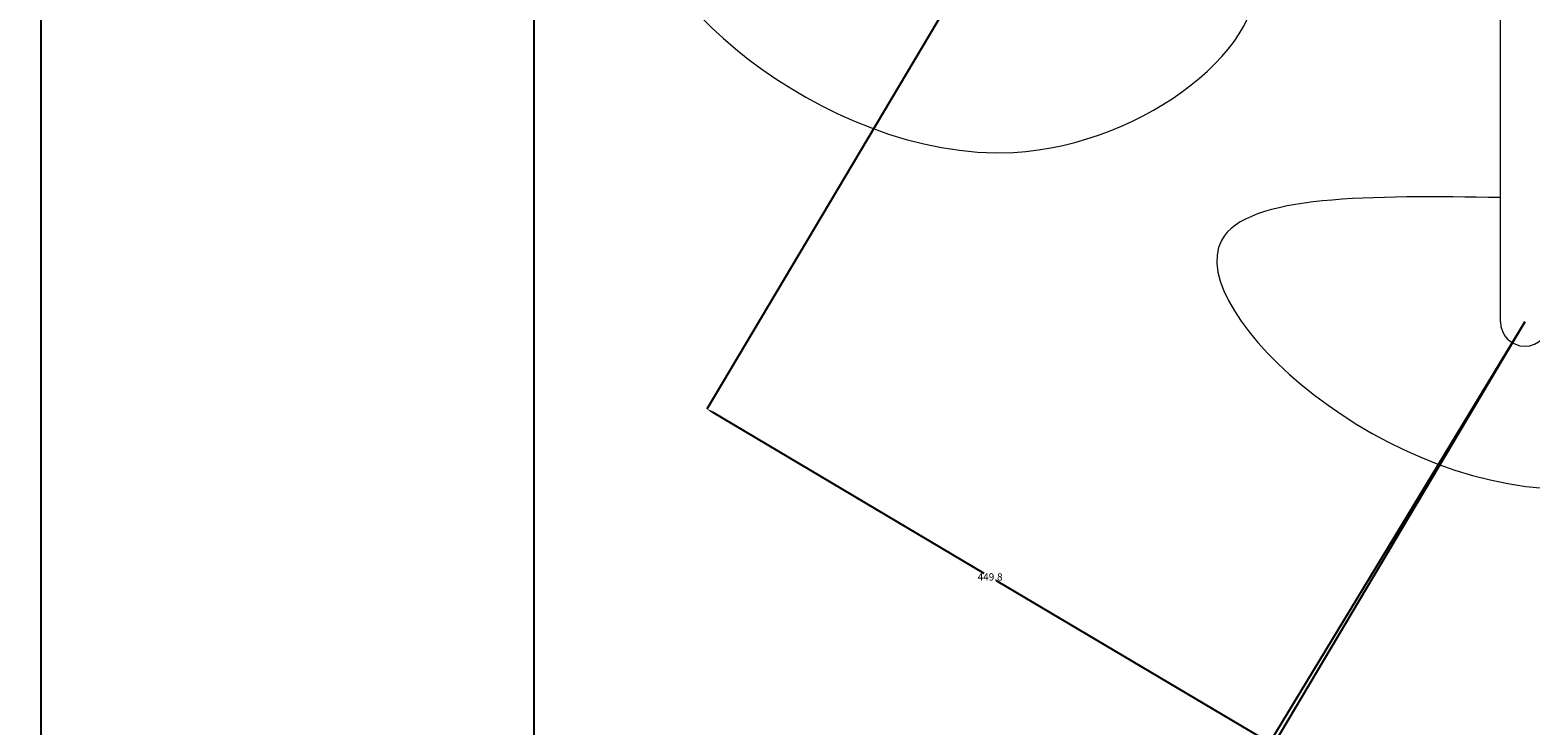
# Model space of a CAD drawing. Units: metres. Extents: x -2391 to 4922, y -635 to 4845.
# Tile 2 of 37: x -2391 to -1367, y 53 to 528. Entities that reach past the tile are written whole.
import ezdxf

# ---------------------------------------------------------------- set-up
doc = ezdxf.new("R2010")
doc.units = ezdxf.units.M
doc.header["$MEASUREMENT"] = 0
doc.layers.add('A-ANNO-DIMS', color=2, linetype='Continuous', lineweight=18)
doc.layers.add('A-FURN', color=8, linetype='Continuous', lineweight=18)
doc.styles.get("Standard").update_dxf_attribs({"font": 'arial.ttf'})
doc.dimstyles.get("Standard").update_dxf_attribs({"dimtxt": 5, "dimasz": 4, "dimexe": 0.18, "dimexo": 0.0625, "dimgap": 0.09, "dimtad": 0, "dimtih": 1, "dimtoh": 1, "dimdec": 0, "dimzin": 0, "dimdsep": 46, "dimtxsty": 'Standard', "dimcen": 0.09, "dimadec": 0, "dimazin": 0, "dimtfac": 1, "dimtdec": 0, "dimtofl": 0, "dimtmove": 0, "dimatfit": 3, "dimfxl": 1, "dimtolj": 1, "dimtzin": 0, "dimarcsym": 0})

# ---------------------------------------------------------------- blocks, each defined once
blk = doc.blocks.new('STOOL-BAR')
for p, q in [((193.7, 114.2), (193.7, 537.3)), ((227.2, 541.6), (227.2, 114.2))]:
    blk.add_line(p, q)
blk.add_arc((210.4, 114.2), 16.7, 180, 0)
for points, knots in [([(47.2, 931.3), (26.8, 772.8), (-15.6, 443.8), (639.9, 614.2), (403.7, 766.2), (59.9, 548.3), (308.4, 1061), (87.9, 1049.3), (63.7, 979.1), (47.2, 931.3)], [0, 0, 0, 0, 373.373325, 775.091582, 839.205201, 1103.589215, 1452.822506, 1516.235646, 1651.960559, 1651.960559, 1651.960559, 1651.960559]), ([(82.7, 605.1), (79.4, 599.1), (25.4, 501.4), (205.2, 535.3), (373.8, 567.1)], [0, 0, 0, 0, 19.816883, 320.720948, 320.720948, 320.720948, 320.720948]), ([(193.7, 199.1), (106.9, 200.3), (-113.9, 203.4), (215.4, -95.9), (508.4, 143.5), (296.5, 208.8), (227.2, 200.8)], [0, 0, 0, 0, 131.596892, 334.838301, 476.929251, 613.088937, 613.088937, 613.088937, 613.088937])]:
    blk.add_open_spline(points, degree=3, knots=knots)
blk = doc.blocks.new('*D8')
at = {"layer": 'A-ANNO-DIMS', "color": 0, "lineweight": -2, "transparency": 16777216}
for p, q in [((-2047.3, 3005.2), (-2047.3, -631.4)), ((4577.8, 2350.2), (4577.8, -631.4)), ((-2043.3, -631.2), (1257.6, -631.2)), ((4573.8, -631.2), (1272.8, -631.2))]:
    blk.add_line(p, q, dxfattribs=at)
at = {"layer": 'A-ANNO-DIMS', "color": 0, "transparency": 16777216}
for points in [[(-2043.3, -630.6), (-2043.3, -631.9), (-2047.3, -631.2)], [(4573.8, -630.6), (4573.8, -631.9), (4577.8, -631.2)]]:
    blk.add_solid(points, dxfattribs=at)
at = {"layer": 'Defpoints', "color": 0, "transparency": 16777216}
for p in [(-2047.3, 3005.3), (4577.8, 2350.3), (4577.8, -631.2)]:
    blk.add_point(p, dxfattribs=at)
at = {"layer": 'A-ANNO-DIMS', "color": 0, "transparency": 16777216, "insert": (1265.2, -631.2), "char_height": 5, "attachment_point": 5}
blk.add_mtext('\\A1;6625', dxfattribs=at)
blk = doc.blocks.new('*D10')
at = {"layer": 'A-ANNO-DIMS', "color": 0, "lineweight": -2, "transparency": 16777216}
for p, q in [((550.7, 4505.3), (-2384, 4505.3)), ((-2383.8, 4501.3), (-2383.8, 2107.9)), ((-2383.8, -290.7), (-2383.8, 2102.6)), ((-488.6, -294.7), (-2384, -294.7))]:
    blk.add_line(p, q, dxfattribs=at)
at = {"layer": 'A-ANNO-DIMS', "color": 0, "transparency": 16777216}
for points in [[(-2384.5, 4501.3), (-2383.2, 4501.3), (-2383.8, 4505.3)], [(-2384.5, -290.7), (-2383.2, -290.7), (-2383.8, -294.7)]]:
    blk.add_solid(points, dxfattribs=at)
at = {"layer": 'Defpoints', "color": 0, "transparency": 16777216}
for p in [(-2383.8, 4505.3), (550.7, 4505.3), (-488.5, -294.7)]:
    blk.add_point(p, dxfattribs=at)
at = {"layer": 'A-ANNO-DIMS', "color": 0, "transparency": 16777216, "insert": (-2383.8, 2105.3), "char_height": 5, "attachment_point": 5}
blk.add_mtext('\\A1;4800', dxfattribs=at)
blk = doc.blocks.new('*D50')
at = {"layer": 'A-ANNO-DIMS', "color": 0, "lineweight": -2, "transparency": 16777216}
for p, q in [((-1757.3, 558), (-1929.2, 268.6)), ((-1370.5, 328.3), (-1542.4, 38.9)), ((-1925.6, 266.7), (-1740.1, 156.5)), ((-1545.8, 41.1), (-1731.3, 151.2))]:
    blk.add_line(p, q, dxfattribs=at)
at = {"layer": 'A-ANNO-DIMS', "color": 0, "transparency": 16777216}
for points in [[(-1925.3, 267.3), (-1926, 266.1), (-1929.1, 268.7)], [(-1545.4, 41.6), (-1546.1, 40.5), (-1542.3, 39)]]:
    blk.add_solid(points, dxfattribs=at)
at = {"layer": 'Defpoints', "color": 0, "transparency": 16777216}
for p in [(-1757.2, 558.1), (-1370.5, 328.3), (-1929.1, 268.7)]:
    blk.add_point(p, dxfattribs=at)
at = {"layer": 'A-ANNO-DIMS', "color": 0, "transparency": 16777216, "insert": (-1735.7, 153.9), "char_height": 5, "attachment_point": 5}
blk.add_mtext('\\A1;449.8', dxfattribs=at)
blk = doc.blocks.new('*D51')
at = {"layer": 'A-ANNO-DIMS', "color": 0, "lineweight": -2, "transparency": 16777216}
for p, q in [((-1370.5, 328.3), (-1544.9, 40.4)), ((-1541.4, 38.4), (-1301.9, -106.6)), ((-876, 28.7), (-1050.4, -259.2)), ((-1053.8, -257), (-1293.2, -111.9))]:
    blk.add_line(p, q, dxfattribs=at)
at = {"layer": 'A-ANNO-DIMS', "color": 0, "transparency": 16777216}
for points in [[(-1541.1, 39), (-1541.8, 37.9), (-1544.8, 40.5)], [(-1053.4, -256.4), (-1054.1, -257.5), (-1050.3, -259)]]:
    blk.add_solid(points, dxfattribs=at)
at = {"layer": 'Defpoints', "color": 0, "transparency": 16777216}
for p in [(-1370.5, 328.3), (-1544.8, 40.5), (-876, 28.8)]:
    blk.add_point(p, dxfattribs=at)
at = {"layer": 'A-ANNO-DIMS', "color": 0, "transparency": 16777216, "insert": (-1297.6, -109.3), "char_height": 5, "attachment_point": 5}
blk.add_mtext('\\A1;578.1', dxfattribs=at)

msp = doc.modelspace()

# ---------------------------------------------------------------- linework, layer by layer
at = {"layer": 'A-FURN'}
msp.add_open_spline([(-1773.9741, 642.9857), (-1860.7418, 644.1794), (-2081.5157, 647.2169), (-1752.1913, 347.944), (-1459.2678, 587.3777), (-1671.1165, 652.6299), (-1740.4832, 644.6157)], degree=3, knots=[0, 0, 0, 0, 131.596891544, 334.838301031, 476.929251308, 613.088936904, 613.088936904, 613.088936904, 613.088936904], dxfattribs=at)

# ---------------------------------------------------------------- block references
msp.add_blockref('STOOL-BAR', (-1580.882, 214.116), dxfattribs=at)

# ---------------------------------------------------------------- dimensions: what is measured, and where the dimension line sits
at = {"layer": 'A-ANNO-DIMS'}
for base, p1, p2, angle, override, picture, middle in [((-2383.8343, 4505.2763), (-488.4886, -294.7237), (550.7419, 4505.2763), 90, {"dimdec": 0, "dimlfac": 1, "dimrnd": 0, "dimzin": 0, "dimdsep": 46, "dimlunit": 2}, '*D10', (-2383.8343, 2105.2763)), ((-1929.0761, 268.7454), (-1370.4753, 328.3288), (-1757.2287, 558.0561), 149.2901447, {"dimdec": 1, "dimlfac": 1, "dimrnd": 0, "dimzin": 0, "dimdsep": 46, "dimlunit": 2}, '*D50', (-1735.6994, 153.8817)), ((-1544.828, 40.5209), (-875.9874, 28.7702), (-1370.4753, 328.3288), 148.7927031, {"dimdec": 1, "dimlfac": 1, "dimrnd": 0, "dimzin": 0, "dimdsep": 46, "dimlunit": 2}, '*D51', (-1297.5841, -109.2584))]:
    dim = msp.add_linear_dim(base=base, p1=p1, p2=p2, angle=angle, dimstyle='Standard', override=override, dxfattribs=at)
    dim.commit()
    dim.dimension.update_dxf_attribs({"geometry": picture, "text_midpoint": middle})
dim = msp.add_linear_dim(base=(4577.76, -631.2237), p1=(-2047.3343, 3005.2763), p2=(4577.76, 2350.2763), dimstyle='Standard', override={"dimdec": 0, "dimlfac": 1, "dimrnd": 0, "dimzin": 0, "dimdsep": 46, "dimlunit": 2}, dxfattribs=at)
dim.commit()
dim.dimension.update_dxf_attribs({"geometry": '*D8', "text_midpoint": (1265.2128, -631.2237)})

doc.saveas('drawing.dxf')
